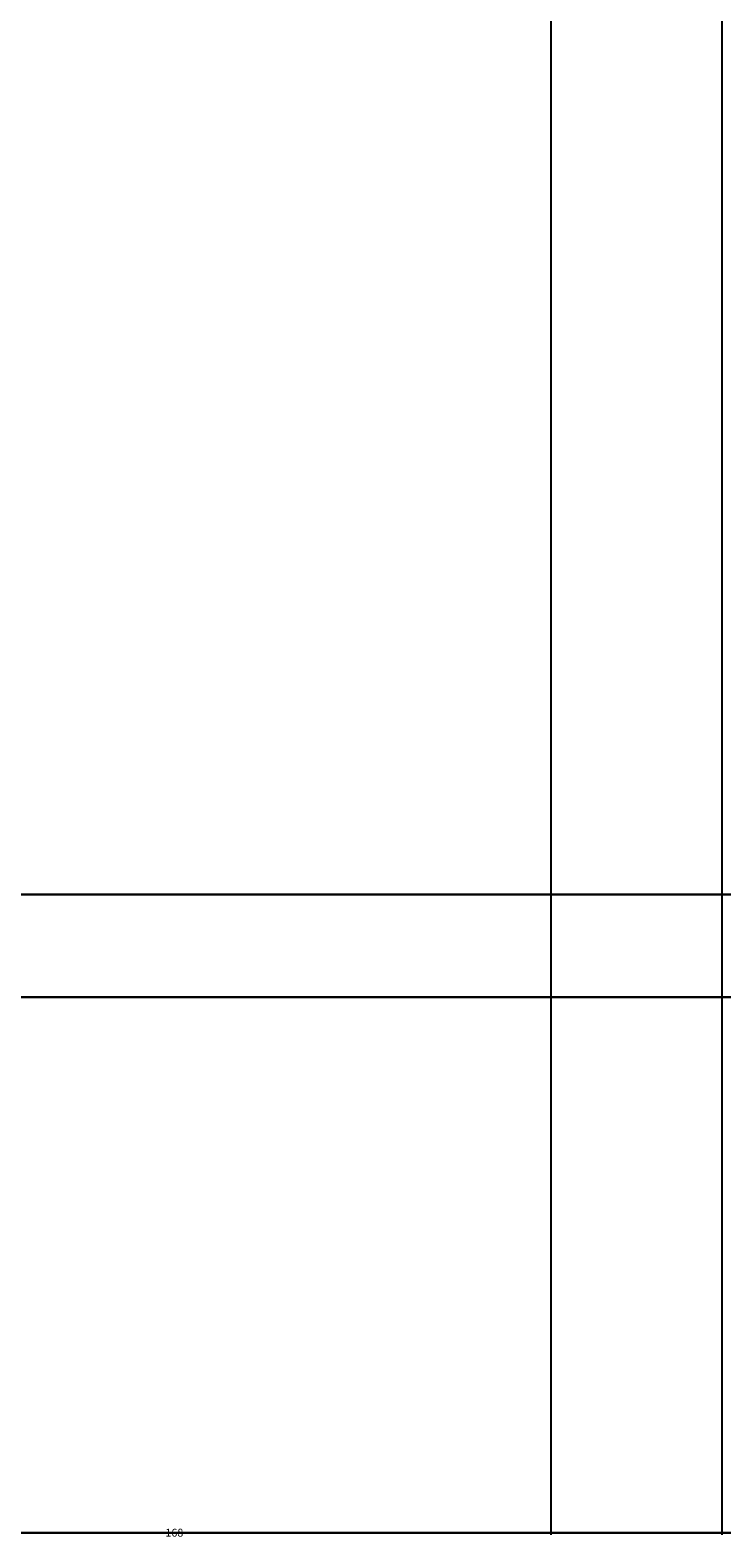
# Model space of a CAD drawing. Units: inches. Extents: x 867 to 1667, y -234 to 788.
# Tile 5 of 42: x 1151 to 1212, y -234 to -102. Entities that reach past the tile are written whole.
import ezdxf

# ---------------------------------------------------------------- set-up
doc = ezdxf.new("R2010")
doc.units = ezdxf.units.IN
doc.header["$MEASUREMENT"] = 0
doc.layers.add('A-ANNO-DIMS', color=2, linetype='Continuous', lineweight=18)
doc.layers.add('A-WALL-SITE', color=8, linetype='Continuous', lineweight=30)
doc.styles.get("Standard").update_dxf_attribs({"font": 'arial.ttf'})
doc.dimstyles.get("Standard").update_dxf_attribs({"dimtxt": 0.6875, "dimasz": 0.18, "dimexe": 0.18, "dimexo": 0.0625, "dimgap": 0.09, "dimtad": 0, "dimdec": 4, "dimzin": 0, "dimdsep": 46, "dimlunit": 4, "dimtxsty": 'Standard', "dimcen": 0.09, "dimadec": 0, "dimazin": 0, "dimtfac": 1, "dimtdec": 4, "dimtofl": 0, "dimtmove": 0, "dimatfit": 3, "dimfxl": 1, "dimtolj": 1, "dimtzin": 0, "dimarcsym": 0})

# ---------------------------------------------------------------- blocks, each defined once
blk = doc.blocks.new('*D27')
at = {"layer": 'A-ANNO-DIMS', "color": 0, "lineweight": -2, "transparency": 16777216}
for p, q in [((1070.89, -55.97), (1070.89, -233.54)), ((1525.26, -186.47), (1525.26, -233.54)), ((1071.07, -233.36), (1296.81, -233.36)), ((1525.08, -233.36), (1299.34, -233.36))]:
    blk.add_line(p, q, dxfattribs=at)
at = {"layer": 'A-ANNO-DIMS', "color": 0, "transparency": 16777216}
for points in [[(1071.07, -233.33), (1071.07, -233.39), (1070.89, -233.36)], [(1525.08, -233.33), (1525.08, -233.39), (1525.26, -233.36)]]:
    blk.add_solid(points, dxfattribs=at)
at = {"layer": 'Defpoints', "color": 0, "transparency": 16777216}
for p in [(1070.89, -55.91), (1525.26, -186.41), (1525.26, -233.36)]:
    blk.add_point(p, dxfattribs=at)
at = {"layer": 'A-ANNO-DIMS', "color": 0, "transparency": 16777216, "insert": (1298.08, -233.36), "char_height": 0.688, "attachment_point": 5}
blk.add_mtext('\\A1;454.4', dxfattribs=at)
blk = doc.blocks.new('*D37')
at = {"layer": 'A-ANNO-DIMS', "color": 0, "lineweight": -2, "transparency": 16777216}
for p, q in [((1049.89, 257.55), (1049.89, -233.54)), ((1196.89, 257.55), (1196.89, -233.54)), ((1050.07, -233.36), (1122.57, -233.36)), ((1196.71, -233.36), (1124.2, -233.36))]:
    blk.add_line(p, q, dxfattribs=at)
at = {"layer": 'A-ANNO-DIMS', "color": 0, "transparency": 16777216}
for points in [[(1050.07, -233.33), (1050.07, -233.39), (1049.89, -233.36)], [(1196.71, -233.33), (1196.71, -233.39), (1196.89, -233.36)]]:
    blk.add_solid(points, dxfattribs=at)
at = {"layer": 'Defpoints', "color": 0, "transparency": 16777216}
for p in [(1049.89, 257.62), (1196.89, 257.62), (1196.89, -233.36)]:
    blk.add_point(p, dxfattribs=at)
at = {"layer": 'A-ANNO-DIMS', "color": 0, "transparency": 16777216, "insert": (1123.39, -233.36), "char_height": 0.688, "attachment_point": 5}
blk.add_mtext('\\A1;147', dxfattribs=at)
blk = doc.blocks.new('*D45')
at = {"layer": 'A-ANNO-DIMS', "color": 0, "lineweight": -2, "transparency": 16777216}
for p, q in [((1079.89, -7.95), (1079.89, -233.54)), ((1247.89, -7.95), (1247.89, -233.54)), ((1080.07, -233.36), (1163.07, -233.36)), ((1247.71, -233.36), (1164.7, -233.36))]:
    blk.add_line(p, q, dxfattribs=at)
at = {"layer": 'A-ANNO-DIMS', "color": 0, "transparency": 16777216}
for points in [[(1080.07, -233.33), (1080.07, -233.39), (1079.89, -233.36)], [(1247.71, -233.33), (1247.71, -233.39), (1247.89, -233.36)]]:
    blk.add_solid(points, dxfattribs=at)
at = {"layer": 'Defpoints', "color": 0, "transparency": 16777216}
for p in [(1079.89, -7.88), (1247.89, -7.88), (1247.89, -233.36)]:
    blk.add_point(p, dxfattribs=at)
at = {"layer": 'A-ANNO-DIMS', "color": 0, "transparency": 16777216, "insert": (1163.89, -233.36), "char_height": 0.688, "attachment_point": 5}
blk.add_mtext('\\A1;168', dxfattribs=at)
blk = doc.blocks.new('*D49')
at = {"layer": 'A-ANNO-DIMS', "color": 0, "lineweight": -2, "transparency": 16777216}
for p, q in [((1070.89, -55.97), (1070.89, -233.54)), ((1211.89, -55.97), (1211.89, -233.54)), ((1071.07, -233.36), (1140.64, -233.36)), ((1211.71, -233.36), (1142.14, -233.36))]:
    blk.add_line(p, q, dxfattribs=at)
at = {"layer": 'A-ANNO-DIMS', "color": 0, "transparency": 16777216}
for points in [[(1071.07, -233.33), (1071.07, -233.39), (1070.89, -233.36)], [(1211.71, -233.33), (1211.71, -233.39), (1211.89, -233.36)]]:
    blk.add_solid(points, dxfattribs=at)
at = {"layer": 'Defpoints', "color": 0, "transparency": 16777216}
for p in [(1070.89, -55.91), (1211.89, -55.91), (1211.89, -233.36)]:
    blk.add_point(p, dxfattribs=at)
at = {"layer": 'A-ANNO-DIMS', "color": 0, "transparency": 16777216, "insert": (1141.39, -233.36), "char_height": 0.688, "attachment_point": 5}
blk.add_mtext('\\A1;141', dxfattribs=at)
blk = doc.blocks.new('*D50')
at = {"layer": 'A-ANNO-DIMS', "color": 0, "lineweight": -2, "transparency": 16777216}
for p, q in [((1211.89, -103.97), (1211.89, -233.54)), ((1427.89, -103.97), (1427.89, -233.54)), ((1212.07, -233.36), (1319.03, -233.36)), ((1427.71, -233.36), (1320.74, -233.36))]:
    blk.add_line(p, q, dxfattribs=at)
at = {"layer": 'A-ANNO-DIMS', "color": 0, "transparency": 16777216}
for points in [[(1212.07, -233.33), (1212.07, -233.39), (1211.89, -233.36)], [(1427.71, -233.33), (1427.71, -233.39), (1427.89, -233.36)]]:
    blk.add_solid(points, dxfattribs=at)
at = {"layer": 'Defpoints', "color": 0, "transparency": 16777216}
for p in [(1211.89, -103.91), (1427.89, -103.91), (1427.89, -233.36)]:
    blk.add_point(p, dxfattribs=at)
at = {"layer": 'A-ANNO-DIMS', "color": 0, "transparency": 16777216, "insert": (1319.89, -233.36), "char_height": 0.688, "attachment_point": 5}
blk.add_mtext('\\A1;216', dxfattribs=at)

msp = doc.modelspace()

# ---------------------------------------------------------------- linework, layer by layer
at = {"layer": 'A-WALL-SITE'}
for p, q in [((1526.8389, -177.4081), (1006.3882, -177.4081)), ((1619.8866, -186.4081), (914.8866, -186.4081))]:
    msp.add_line(p, q, dxfattribs=at)

# ---------------------------------------------------------------- dimensions: what is measured, and where the dimension line sits
at = {"layer": 'A-ANNO-DIMS'}
for base, p1, p2, override, picture, middle in [((1196.8866, -233.3581), (1049.8866, 257.617), (1196.8866, 257.617), {"dimdec": 0, "dimlfac": 1, "dimrnd": 0, "dimzin": 0, "dimdsep": 46, "dimlunit": 2}, '*D37', (1123.3866, -233.3581)), ((1247.8866, -233.3581), (1079.8866, -7.883), (1247.8866, -7.883), {"dimdec": 0, "dimlfac": 1, "dimrnd": 0, "dimzin": 0, "dimdsep": 46, "dimlunit": 2}, '*D45', (1163.8866, -233.3581)), ((1525.2648, -233.3581), (1070.8866, -55.9081), (1525.2648, -186.4081), {"dimdec": 1, "dimlfac": 1, "dimrnd": 0, "dimzin": 0, "dimdsep": 46, "dimlunit": 2}, '*D27', (1298.0757, -233.3581)), ((1211.8866, -233.3581), (1070.8866, -55.9081), (1211.8866, -55.9081), {"dimdec": 0, "dimlfac": 1, "dimrnd": 0, "dimzin": 0, "dimdsep": 46, "dimlunit": 2}, '*D49', (1141.3866, -233.3581)), ((1427.8866, -233.3581), (1211.8866, -103.9081), (1427.8866, -103.9081), {"dimdec": 0, "dimlfac": 1, "dimrnd": 0, "dimzin": 0, "dimdsep": 46, "dimlunit": 2}, '*D50', (1319.8866, -233.3581))]:
    dim = msp.add_linear_dim(base=base, p1=p1, p2=p2, dimstyle='Standard', override=override, dxfattribs=at)
    dim.commit()
    dim.dimension.update_dxf_attribs({"geometry": picture, "text_midpoint": middle})

doc.saveas('drawing.dxf')
